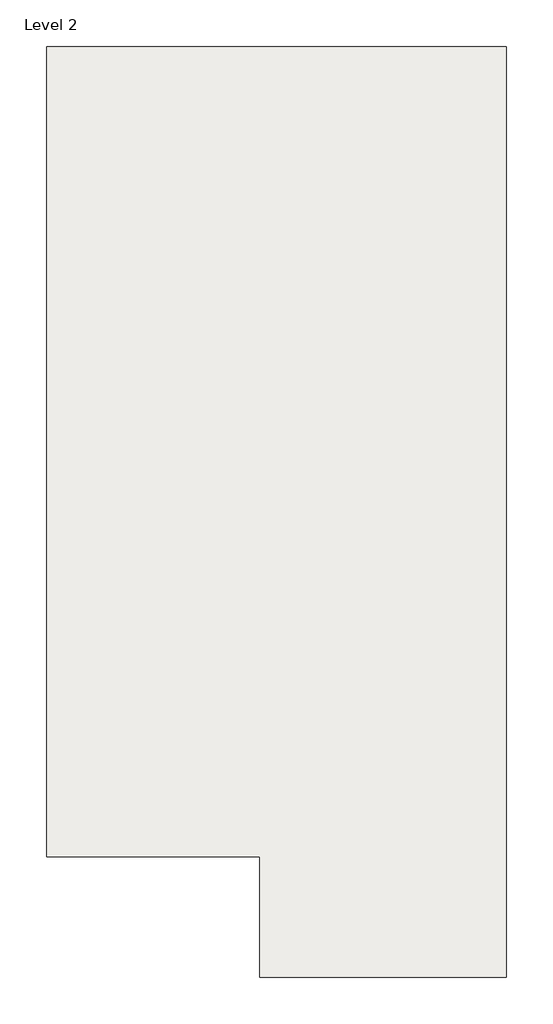
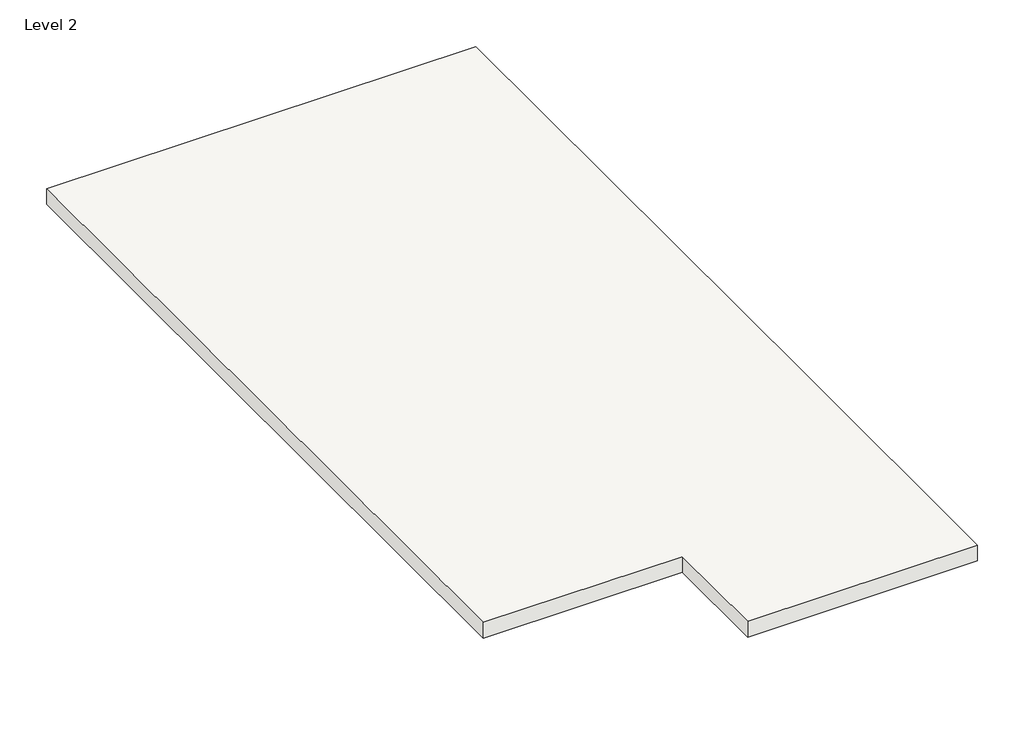
# One storey: 1 roof.
"""IFC4 building model written with IfcOpenShell, lengths in millimetres."""

from ifc_helpers import new_model, si_unit, frame, origin, place, context, project, spatial, polyline, outline, extrude, element, save

model = new_model("IFC4")

# Units and contexts
model_context = context("Model", 3, world=origin())
ifc_project = project(units=[si_unit("LENGTHUNIT", "METRE", prefix="MILLI")], contexts=[model_context])

# Site, building, storey
site = spatial("IfcSite", under=ifc_project)
building = spatial("IfcBuilding", under=site)
storey = spatial("IfcBuildingStorey", under=building, Name="Level 2", Elevation=3048.0)

# Roof
placement = place(None, origin())
element("IfcRoof", 1, ObjectType="Generic - 12\"", at=placement, inside=storey, context=model_context, shape_type="SweptSolid", body=[
    extrude(outline(polyline([(-3091.5660284, 10679.050395), (4731.6339716, 10679.050395), (4731.6339716, 239.650395), (4731.6339716, -5170.549605), (540.6339716, -5170.549605), (540.6339716, -3113.149605), (-3091.5660284, -3113.149605), (-3091.5660284, 10679.050395)])), frame((0.0, 0.0, 3048.0), z_axis=(0.0, 0.0, 1.0), x_axis=(1.0, 0.0, 0.0)), (0.0, 0.0, 1.0), 304.8),
])

save(model, "model.ifc")

# Revit data of these elements
# Type "Generic - 12\""
#   Assembly Code = "B1020"
#   Layers, outside or top first: 1' - 0" "Brick, Soldier Course" (function 1)
# Element 1 (IfcRoof, "Generic - 12\"")
#   built-in parameter 1001705 = 11 (stored number, unit not read)
#   built-in parameter 1001710 = 33615
#   Phase Created = New Construction
#   Materials on its faces: "Brick, Soldier Course"
# Materials
#   "Brick, Soldier Course": class "Masonry", colour RGB 170 98 104, transparency 0, Description = "Common brick soldier coursed", Cost = 0
